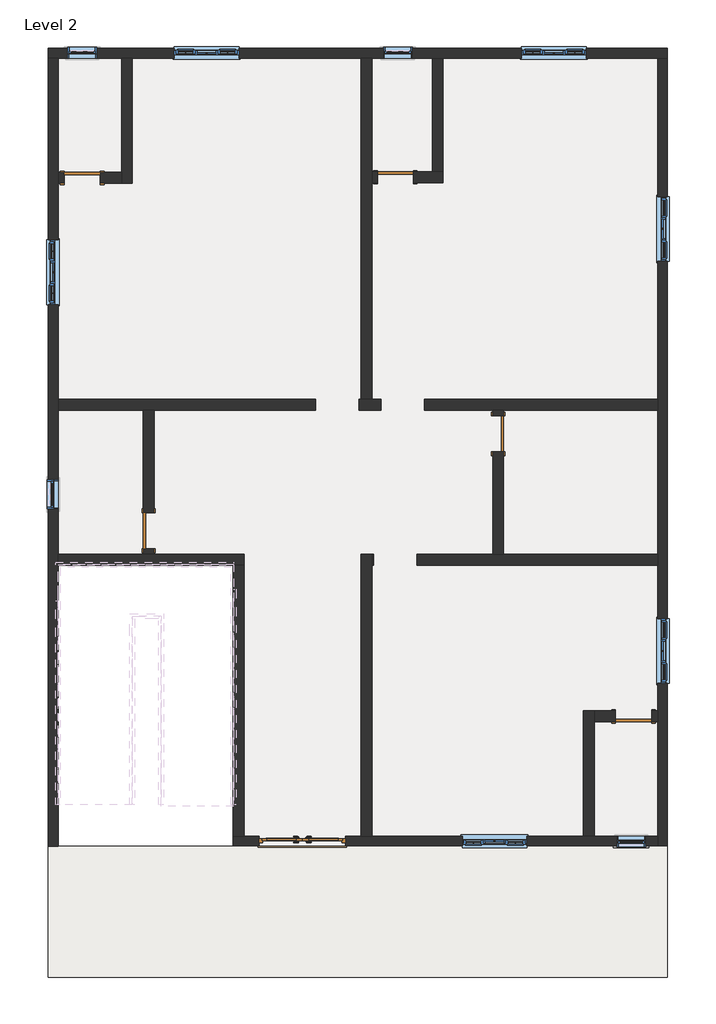
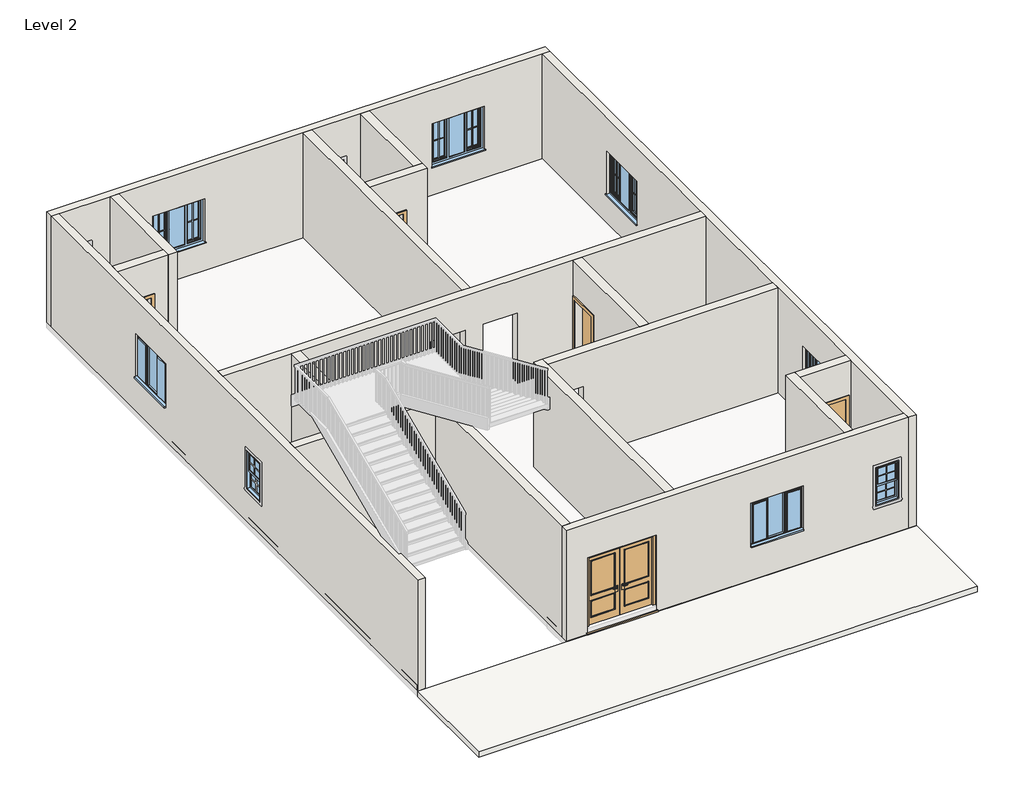
# One storey, part 1 of 4: 18 walls, 10 windows, 6 doors, 1 slab.
"""IFC4 building model written with IfcOpenShell, lengths in millimetres."""

from ifc_helpers import new_model, si_unit, frame, origin, place, context, project, spatial, polyline, outline, extrude, faceted_brep, transform, mapped, element, save
from components import doors_extdbl_2_1810x2110mm_9ab1935a, doors_extdbl_2_1810x2110mm_b7024f51, door_85036156, window_679d2811, windows_tpl_w_glazing_cross_bars_1360x1210mm_0306471f

model = new_model("IFC4")

# Units and contexts
model_context = context("Model", 3, world=origin())
ifc_project = project(units=[si_unit("LENGTHUNIT", "METRE", prefix="MILLI")], contexts=[model_context])

# Site, building, storey
site = spatial("IfcSite", under=ifc_project)
building = spatial("IfcBuilding", under=site)
storey = spatial("IfcBuildingStorey", under=building, Name="Level 2", Elevation=3048.0)

# Doors
placement = place(None, origin())
doors_extdbl_2_1810x2110mm_shape = doors_extdbl_2_1810x2110mm_9ab1935a(model_context)
doors_extdbl_2_1810x2110mm_2_shape = doors_extdbl_2_1810x2110mm_b7024f51(model_context)
element("IfcDoor", 1, ObjectType="Doors_ExtDbl_2 : 1810x2110mm", at=placement, inside=storey, context=model_context, shape_type="MappedRepresentation", body=[
    mapped(doors_extdbl_2_1810x2110mm_shape, transform((-2421.0852725, -7729.5064015, 3048.0), x_axis=(1.0, 0.0, 0.0), y_axis=(0.0, 1.0, 0.0), z_axis=(0.0, 0.0, 1.0))),
    mapped(doors_extdbl_2_1810x2110mm_2_shape, transform((-2421.0852725, -7729.5064015, 3048.0), x_axis=(1.0, 0.0, 0.0), y_axis=(0.0, 1.0, 0.0), z_axis=(0.0, 0.0, 1.0))),
])
door_shape = door_85036156(model_context)
element("IfcDoor", 2, ObjectType="Single-Flush : 30\" x 80\"", at=placement, inside=storey, context=model_context, shape_type="MappedRepresentation", body=[
    mapped(door_shape, transform((-7046.4415084, 6189.6935985, 3048.0), x_axis=(-1.0, 0.0, 0.0), y_axis=(0.0, -1.0, 0.0), z_axis=(0.0, 0.0, 1.0))),
])
element("IfcDoor", 3, ObjectType="Single-Flush : 30\" x 80\"", at=placement, inside=storey, context=model_context, shape_type="MappedRepresentation", body=[
    mapped(door_shape, transform((-467.8415084, 6203.2000968, 3048.0), x_axis=(-1.0, 0.0, 0.0), y_axis=(0.0, -1.0, 0.0), z_axis=(0.0, 0.0, 1.0))),
])
element("IfcDoor", 4, ObjectType="Single-Flush : 30\" x 80\"", at=placement, inside=storey, context=model_context, shape_type="MappedRepresentation", body=[
    mapped(door_shape, transform((-5649.4415084, -1217.2217109, 3048.0), x_axis=(0.0, -1.0, 0.0), y_axis=(1.0, 0.0, 0.0), z_axis=(0.0, 0.0, 1.0))),
])
element("IfcDoor", 5, ObjectType="Single-Flush : 30\" x 80\"", at=placement, inside=storey, context=model_context, shape_type="MappedRepresentation", body=[
    mapped(door_shape, transform((1691.1584916, 817.5935985, 3048.0), x_axis=(0.0, 1.0, 0.0), y_axis=(-1.0, 0.0, 0.0), z_axis=(0.0, 0.0, 1.0))),
])
element("IfcDoor", 6, ObjectType="Single-Flush : 30\" x 80\"", at=placement, inside=storey, context=model_context, shape_type="MappedRepresentation", body=[
    mapped(door_shape, transform((4535.9584916, -5113.3064015, 3048.0), x_axis=(1.0, 0.0, 0.0), y_axis=(0.0, 1.0, 0.0), z_axis=(0.0, 0.0, 1.0))),
])

# Slab
element("IfcSlab", 7, ObjectType="Generic - 12\"", at=placement, inside=storey, context=model_context, shape_type="SweptSolid", body=[
    extrude(outline(polyline([(5247.1584916, -7843.8064015), (5247.1584916, -10593.3139891), (-7757.6415084, -10593.3139891), (-7757.6415084, -7843.8064015), (5247.1584916, -7843.8064015)])), frame((0.0, 0.0, 2895.6), z_axis=(0.0, 0.0, 1.0), x_axis=(1.0, 0.0, 0.0)), (0.0, 0.0, 1.0), 152.4),
])

# Walls
element("IfcWall", 8, ObjectType="Generic - 4.5\"", at=placement, inside=storey, context=model_context, shape_type="Brep", body=[
    faceted_brep([(-1232.0415084, 1312.8935985, 5158.0), (-1232.0415084, 1312.8935985, 3048.0), (-770.4415084, 1312.8935985, 3048.0), (-770.4415084, 1312.8935985, 5158.0), (139.5584916, 1312.8935985, 5158.0), (139.5584916, 1312.8935985, 3048.0), (1576.8584916, 1312.8935985, 3048.0), (1805.4584916, 1312.8935985, 3048.0), (5043.9584916, 1312.8935985, 3048.0), (5043.9584916, 1312.8935985, 6096.0), (1805.4584916, 1312.8935985, 6096.0), (1576.8584916, 1312.8935985, 6096.0), (-5535.1415084, 1312.8935985, 6096.0), (-5763.7415084, 1312.8935985, 6096.0), (-7554.4415084, 1312.8935985, 6096.0), (-7554.4415084, 1312.8935985, 3048.0), (-5763.7415084, 1312.8935985, 3048.0), (-5535.1415084, 1312.8935985, 3048.0), (-2142.0415084, 1312.8935985, 3048.0), (-2142.0415084, 1312.8935985, 5158.0), (-770.4415084, 1541.4935985, 3048.0), (-963.1415084, 1541.4935985, 3048.0), (-1191.7415084, 1541.4935985, 3048.0), (-1232.0415084, 1541.4935985, 3048.0), (-1232.0415084, 1541.4935985, 5158.0), (-2142.0415084, 1541.4935985, 5158.0), (-2142.0415084, 1541.4935985, 3048.0), (-7554.4415084, 1541.4935985, 3048.0), (-7554.4415084, 1541.4935985, 6096.0), (-1191.7415084, 1541.4935985, 6096.0), (-963.1415084, 1541.4935985, 6096.0), (5043.9584916, 1541.4935985, 6096.0), (5043.9584916, 1541.4935985, 3048.0), (139.5584916, 1541.4935985, 3048.0), (139.5584916, 1541.4935985, 5158.0), (-770.4415084, 1541.4935985, 5158.0)], [[[0, 1, 2, 3, 4, 5, 6, 7, 8, 9, 10, 11, 12, 13, 14, 15, 16, 17, 18, 19]], [[20, 21, 22, 23, 24, 25, 26, 27, 28, 29, 30, 31, 32, 33, 34, 35]], [[33, 32, 8, 7, 6, 5]], [[2, 1, 23, 22, 21, 20]], [[18, 17, 16, 15, 27, 26]], [[14, 13, 12, 11, 10, 9, 31, 30, 29, 28]], [[9, 8, 32, 31]], [[15, 14, 28, 27]], [[5, 4, 34, 33]], [[3, 2, 20, 35]], [[4, 3, 35, 34]], [[26, 25, 19, 18]], [[24, 23, 1, 0]], [[25, 24, 0, 19]]]),
])
element("IfcWall", 9, ObjectType="Generic - 4.5\"", at=placement, inside=storey, context=model_context, shape_type="Brep", body=[
    faceted_brep([(-1191.7415084, 8704.2935985, 3048.0), (-1191.7415084, 1541.4935985, 3048.0), (-1191.7415084, 1541.4935985, 6096.0), (-1191.7415084, 8704.2935985, 6096.0), (-963.1415084, 8704.2935985, 3048.0), (-963.1415084, 8704.2935985, 6096.0), (-963.1415084, 6317.5000968, 6096.0), (-963.1415084, 6088.9000968, 6096.0), (-963.1415084, 1541.4935985, 6096.0), (-963.1415084, 1541.4935985, 3048.0), (-963.1415084, 6088.9000968, 3048.0), (-963.1415084, 6317.5000968, 3048.0)], [[[0, 1, 2, 3]], [[4, 5, 6, 7, 8, 9, 10, 11]], [[1, 0, 4, 11, 10, 9]], [[3, 2, 8, 7, 6, 5]], [[0, 3, 5, 4]], [[2, 1, 9, 8]]]),
])
element("IfcWall", 10, ObjectType="Generic - 4.5\"", at=placement, inside=storey, context=model_context, shape_type="Brep", body=[
    faceted_brep([(-6220.9415084, 8704.2935985, 3048.0), (-6220.9415084, 6303.9935985, 3048.0), (-6220.9415084, 6075.3935985, 3048.0), (-6220.9415084, 6075.3935985, 6096.0), (-6220.9415084, 6303.9935985, 6096.0), (-6220.9415084, 8704.2935985, 6096.0), (-5992.3415084, 8704.2935985, 3048.0), (-5992.3415084, 8704.2935985, 6096.0), (-5992.3415084, 6075.3935985, 6096.0), (-5992.3415084, 6075.3935985, 3048.0)], [[[0, 1, 2, 3, 4, 5]], [[6, 7, 8, 9]], [[2, 1, 0, 6, 9]], [[5, 4, 3, 8, 7]], [[0, 5, 7, 6]], [[3, 2, 9, 8]]]),
])
element("IfcWall", 11, ObjectType="Generic - 4.5\"", at=placement, inside=storey, context=model_context, shape_type="SweptSolid", body=[
    extrude(outline(polyline([(3048.0, -7554.4415084), (3048.0, -7427.4415084), (5080.0, -7427.4415084), (5080.0, -6665.4415084), (3048.0, -6665.4415084), (3048.0, -6220.9415084), (6096.0, -6220.9415084), (6096.0, -7554.4415084), (3048.0, -7554.4415084)])), frame((0.0, 6075.3935985, 0.0), z_axis=(0.0, 1.0, 0.0), x_axis=(0.0, 0.0, 1.0)), (0.0, 0.0, 1.0), 228.6),
])
element("IfcWall", 12, ObjectType="Generic - 4.5\"", at=placement, inside=storey, context=model_context, shape_type="Brep", body=[
    faceted_brep([(-963.1415084, 6088.9000968, 3048.0), (-848.8415084, 6088.9000968, 3048.0), (-848.8415084, 6088.9000968, 5080.0), (-86.8415084, 6088.9000968, 5080.0), (-86.8415084, 6088.9000968, 3048.0), (535.4584916, 6088.9000968, 3048.0), (535.4584916, 6088.9000968, 6096.0), (-963.1415084, 6088.9000968, 6096.0), (-848.8415084, 6317.5000968, 5080.0), (-848.8415084, 6317.5000968, 3048.0), (-963.1415084, 6317.5000968, 3048.0), (-963.1415084, 6317.5000968, 6096.0), (306.8584916, 6317.5000968, 6096.0), (535.4584916, 6317.5000968, 6096.0), (535.4584916, 6317.5000968, 3048.0), (306.8584916, 6317.5000968, 3048.0), (-86.8415084, 6317.5000968, 3048.0), (-86.8415084, 6317.5000968, 5080.0)], [[[0, 1, 2, 3, 4, 5, 6, 7]], [[8, 9, 10, 11, 12, 13, 14, 15, 16, 17]], [[10, 9, 1, 0]], [[16, 15, 14, 5, 4]], [[7, 6, 13, 12, 11]], [[0, 7, 11, 10]], [[6, 5, 14, 13]], [[2, 1, 9, 8]], [[3, 2, 8, 17]], [[4, 3, 17, 16]]]),
])
element("IfcWall", 13, ObjectType="Generic - 4.5\"", at=placement, inside=storey, context=model_context, shape_type="SweptSolid", body=[
    extrude(outline(polyline([(535.4584916, 8704.2935985), (535.4584916, 6317.5000968), (306.8584916, 6317.5000968), (306.8584916, 8704.2935985), (535.4584916, 8704.2935985)])), frame((0.0, 0.0, 3048.0), z_axis=(0.0, 0.0, 1.0), x_axis=(1.0, 0.0, 0.0)), (0.0, 0.0, 1.0), 3048.0),
])
element("IfcWall", 14, ObjectType="Generic - 4.5\"", at=placement, inside=storey, context=model_context, shape_type="SweptSolid", body=[
    extrude(outline(polyline([(-1598.2217109, 5080.0), (-1598.2217109, 3048.0), (-1712.5217109, 3048.0), (-1712.5217109, 6096.0), (1312.8935985, 6096.0), (1312.8935985, 3048.0), (-836.2217109, 3048.0), (-836.2217109, 5080.0), (-1598.2217109, 5080.0)])), frame((-5763.7415084, 0.0, 0.0), z_axis=(1.0, 0.0, 0.0), x_axis=(0.0, 1.0, 0.0)), (0.0, 0.0, 1.0), 228.6),
])
element("IfcWall", 15, ObjectType="Generic - 4.5\"", at=placement, inside=storey, context=model_context, shape_type="Brep", body=[
    faceted_brep([(-7554.4415084, -1941.1217109, 3048.0), (-3879.0290366, -1941.1217109, 3048.0), (-3650.4290366, -1941.1217109, 3048.0), (-3650.4290366, -1941.1217109, 6096.0), (-3879.0290366, -1941.1217109, 6096.0), (-7554.4415084, -1941.1217109, 6096.0), (-7554.4415084, -1712.5217109, 3048.0), (-7554.4415084, -1712.5217109, 6096.0), (-5763.7415084, -1712.5217109, 6096.0), (-5535.1415084, -1712.5217109, 6096.0), (-3650.4290366, -1712.5217109, 6096.0), (-3650.4290366, -1712.5217109, 3048.0), (-5535.1415084, -1712.5217109, 3048.0), (-5763.7415084, -1712.5217109, 3048.0)], [[[0, 1, 2, 3, 4, 5]], [[6, 7, 8, 9, 10, 11, 12, 13]], [[2, 1, 0, 6, 13, 12, 11]], [[5, 4, 3, 10, 9, 8, 7]], [[0, 5, 7, 6]], [[3, 2, 11, 10]]]),
])
element("IfcWall", 16, ObjectType="Generic - 4.5\"", at=placement, inside=storey, context=model_context, shape_type="SweptSolid", body=[
    extrude(outline(polyline([(-3879.0290366, -7627.9064015), (-3879.0290366, -1941.1217109), (-3650.4290366, -1941.1217109), (-3650.4290366, -7627.9064015), (-3879.0290366, -7627.9064015)])), frame((0.0, 0.0, 3048.0), z_axis=(0.0, 0.0, 1.0), x_axis=(1.0, 0.0, 0.0)), (0.0, 0.0, 1.0), 3048.0),
])
element("IfcWall", 17, ObjectType="Generic - 4.5\"", at=placement, inside=storey, context=model_context, shape_type="SweptSolid", body=[
    extrude(outline(polyline([(1312.8935985, 3048.0), (1198.5935985, 3048.0), (1198.5935985, 5080.0), (436.5935985, 5080.0), (436.5935985, 3048.0), (-1712.5217109, 3048.0), (-1712.5217109, 6096.0), (1312.8935985, 6096.0), (1312.8935985, 3048.0)])), frame((1576.8584916, 0.0, 0.0), z_axis=(1.0, 0.0, 0.0), x_axis=(0.0, 1.0, 0.0)), (0.0, 0.0, 1.0), 228.6),
])
element("IfcWall", 18, ObjectType="Generic - 4.5\"", at=placement, inside=storey, context=model_context, shape_type="Brep", body=[
    faceted_brep([(-963.1415084, -7627.9064015, 3048.0), (-963.1415084, -1941.1217109, 3048.0), (-963.1415084, -1712.5217109, 3048.0), (-963.1415084, -1712.5217109, 6096.0), (-963.1415084, -1941.1217109, 6096.0), (-963.1415084, -7627.9064015, 6096.0), (-1191.7415084, -7627.9064015, 3048.0), (-1191.7415084, -7627.9064015, 6096.0), (-1191.7415084, -1712.5217109, 6096.0), (-1191.7415084, -1712.5217109, 3048.0)], [[[0, 1, 2, 3, 4, 5]], [[6, 7, 8, 9]], [[2, 1, 0, 6, 9]], [[5, 4, 3, 8, 7]], [[0, 5, 7, 6]], [[3, 2, 9, 8]]]),
])
element("IfcWall", 19, ObjectType="Generic - 4.5\"", at=placement, inside=storey, context=model_context, shape_type="Brep", body=[
    faceted_brep([(-922.8415084, -1712.5217109, 5158.0), (-922.8415084, -1712.5217109, 3048.0), (-963.1415084, -1712.5217109, 3048.0), (-963.1415084, -1712.5217109, 6096.0), (1576.8584916, -1712.5217109, 6096.0), (1805.4584916, -1712.5217109, 6096.0), (5043.9584916, -1712.5217109, 6096.0), (5043.9584916, -1712.5217109, 3048.0), (1805.4584916, -1712.5217109, 3048.0), (1576.8584916, -1712.5217109, 3048.0), (-12.8415084, -1712.5217109, 3048.0), (-12.8415084, -1712.5217109, 5158.0), (-963.1415084, -1941.1217109, 3048.0), (-922.8415084, -1941.1217109, 3048.0), (-922.8415084, -1941.1217109, 5158.0), (-12.8415084, -1941.1217109, 5158.0), (-12.8415084, -1941.1217109, 3048.0), (5043.9584916, -1941.1217109, 3048.0), (5043.9584916, -1941.1217109, 6096.0), (-963.1415084, -1941.1217109, 6096.0)], [[[0, 1, 2, 3, 4, 5, 6, 7, 8, 9, 10, 11]], [[12, 13, 14, 15, 16, 17, 18, 19]], [[2, 1, 13, 12]], [[10, 9, 8, 7, 17, 16]], [[6, 5, 4, 3, 19, 18]], [[3, 2, 12, 19]], [[7, 6, 18, 17]], [[16, 15, 11, 10]], [[14, 13, 1, 0]], [[15, 14, 0, 11]]]),
])
element("IfcWall", 20, ObjectType="Generic - 4.5\"", at=placement, inside=storey, context=model_context, shape_type="Brep", body=[
    faceted_brep([(3710.4584916, -7627.9064015, 3048.0), (3710.4584916, -5227.6064015, 3048.0), (3710.4584916, -4999.0064015, 3048.0), (3710.4584916, -4999.0064015, 6096.0), (3710.4584916, -5227.6064015, 6096.0), (3710.4584916, -7627.9064015, 6096.0), (3481.8584916, -7627.9064015, 3048.0), (3481.8584916, -7627.9064015, 6096.0), (3481.8584916, -4999.0064015, 6096.0), (3481.8584916, -4999.0064015, 3048.0)], [[[0, 1, 2, 3, 4, 5]], [[6, 7, 8, 9]], [[2, 1, 0, 6, 9]], [[5, 4, 3, 8, 7]], [[0, 5, 7, 6]], [[3, 2, 9, 8]]]),
])
element("IfcWall", 21, ObjectType="Generic - 4.5\"", at=placement, inside=storey, context=model_context, shape_type="SweptSolid", body=[
    extrude(outline(polyline([(5080.0, 4916.9584916), (3048.0, 4916.9584916), (3048.0, 5043.9584916), (6096.0, 5043.9584916), (6096.0, 3710.4584916), (3048.0, 3710.4584916), (3048.0, 4154.9584916), (5080.0, 4154.9584916), (5080.0, 4916.9584916)])), frame((0.0, -5227.6064015, 0.0), z_axis=(0.0, 1.0, 0.0), x_axis=(0.0, 0.0, 1.0)), (0.0, 0.0, 1.0), 228.6),
])
element("IfcWall", 22, ObjectType="Generic - 9\"", at=placement, inside=storey, context=model_context, shape_type="Brep", body=[
    faceted_brep([(-7757.6415084, 8704.2935985, 3048.0), (-7554.4415084, 8704.2935985, 3048.0), (-6220.9415084, 8704.2935985, 3048.0), (-5992.3415084, 8704.2935985, 3048.0), (-1191.7415084, 8704.2935985, 3048.0), (-963.1415084, 8704.2935985, 3048.0), (306.8584916, 8704.2935985, 3048.0), (535.4584916, 8704.2935985, 3048.0), (5043.9584916, 8704.2935985, 3048.0), (5247.1584916, 8704.2935985, 3048.0), (5247.1584916, 8704.2935985, 6096.0), (5043.9584916, 8704.2935985, 6096.0), (535.4584916, 8704.2935985, 6096.0), (306.8584916, 8704.2935985, 6096.0), (-963.1415084, 8704.2935985, 6096.0), (-1191.7415084, 8704.2935985, 6096.0), (-5992.3415084, 8704.2935985, 6096.0), (-6220.9415084, 8704.2935985, 6096.0), (-7554.4415084, 8704.2935985, 6096.0), (-7757.6415084, 8704.2935985, 6096.0), (2179.5584916, 8704.2935985, 5172.4), (3539.5584916, 8704.2935985, 5172.4), (3539.5584916, 8704.2935985, 3962.4), (2179.5584916, 8704.2935985, 3962.4), (-5110.2415084, 8704.2935985, 5172.4), (-3750.2415084, 8704.2935985, 5172.4), (-3750.2415084, 8704.2935985, 3962.4), (-5110.2415084, 8704.2935985, 3962.4), (-7351.2415084, 8704.2935985, 5029.2), (-6741.6415084, 8704.2935985, 5029.2), (-6741.6415084, 8704.2935985, 3962.4), (-7351.2415084, 8704.2935985, 3962.4), (-721.8415084, 8704.2935985, 5029.2), (-112.2415084, 8704.2935985, 5029.2), (-112.2415084, 8704.2935985, 3962.4), (-721.8415084, 8704.2935985, 3962.4), (-7757.6415084, 8907.4935985, 3048.0), (-7757.6415084, 8907.4935985, 6096.0), (5247.1584916, 8907.4935985, 6096.0), (5247.1584916, 8907.4935985, 3048.0), (2179.5584916, 8907.4935985, 5172.4), (2179.5584916, 8907.4935985, 3962.4), (3539.5584916, 8907.4935985, 3962.4), (3539.5584916, 8907.4935985, 5172.4), (-5110.2415084, 8907.4935985, 5172.4), (-5110.2415084, 8907.4935985, 3962.4), (-3750.2415084, 8907.4935985, 3962.4), (-3750.2415084, 8907.4935985, 5172.4), (-7351.2415084, 8907.4935985, 5029.2), (-7351.2415084, 8907.4935985, 3962.4), (-6741.6415084, 8907.4935985, 3962.4), (-6741.6415084, 8907.4935985, 5029.2), (-721.8415084, 8907.4935985, 5029.2), (-721.8415084, 8907.4935985, 3962.4), (-112.2415084, 8907.4935985, 3962.4), (-112.2415084, 8907.4935985, 5029.2)], [[[0, 1, 2, 3, 4, 5, 6, 7, 8, 9, 10, 11, 12, 13, 14, 15, 16, 17, 18, 19], [20, 21, 22, 23], [24, 25, 26, 27], [28, 29, 30, 31], [32, 33, 34, 35]], [[36, 37, 38, 39], [40, 41, 42, 43], [44, 45, 46, 47], [48, 49, 50, 51], [52, 53, 54, 55]], [[9, 8, 7, 6, 5, 4, 3, 2, 1, 0, 36, 39]], [[19, 18, 17, 16, 15, 14, 13, 12, 11, 10, 38, 37]], [[10, 9, 39, 38]], [[41, 40, 20, 23]], [[42, 41, 23, 22]], [[43, 42, 22, 21]], [[40, 43, 21, 20]], [[45, 44, 24, 27]], [[46, 45, 27, 26]], [[47, 46, 26, 25]], [[44, 47, 25, 24]], [[49, 48, 28, 31]], [[50, 49, 31, 30]], [[51, 50, 30, 29]], [[48, 51, 29, 28]], [[53, 52, 32, 35]], [[54, 53, 35, 34]], [[55, 54, 34, 33]], [[52, 55, 33, 32]], [[0, 19, 37, 36]]]),
])
element("IfcWall", 23, ObjectType="Generic - 9\"", at=placement, inside=storey, context=model_context, shape_type="Brep", body=[
    faceted_brep([(5043.9584916, 8704.2935985, 3048.0), (5043.9584916, 1541.4935985, 3048.0), (5043.9584916, 1312.8935985, 3048.0), (5043.9584916, -1712.5217109, 3048.0), (5043.9584916, -1941.1217109, 3048.0), (5043.9584916, -4999.0064015, 3048.0), (5043.9584916, -5227.6064015, 3048.0), (5043.9584916, -7627.9064015, 3048.0), (5043.9584916, -7831.1064015, 3048.0), (5043.9584916, -7831.1064015, 6096.0), (5043.9584916, -7627.9064015, 6096.0), (5043.9584916, -5227.6064015, 6096.0), (5043.9584916, -4999.0064015, 6096.0), (5043.9584916, -1941.1217109, 6096.0), (5043.9584916, -1712.5217109, 6096.0), (5043.9584916, 1312.8935985, 6096.0), (5043.9584916, 1541.4935985, 6096.0), (5043.9584916, 8704.2935985, 6096.0), (5043.9584916, 5796.5435985, 5172.4), (5043.9584916, 4436.5435985, 5172.4), (5043.9584916, 4436.5435985, 3962.4), (5043.9584916, 5796.5435985, 3962.4), (5043.9584916, -3061.7064015, 5172.4), (5043.9584916, -4421.7064015, 5172.4), (5043.9584916, -4421.7064015, 3962.4), (5043.9584916, -3061.7064015, 3962.4), (5247.1584916, 8704.2935985, 3048.0), (5247.1584916, 8704.2935985, 6096.0), (5247.1584916, -7831.1064015, 6096.0), (5247.1584916, -7831.1064015, 3048.0), (5247.1584916, 5796.5435985, 5172.4), (5247.1584916, 5796.5435985, 3962.4), (5247.1584916, 4436.5435985, 3962.4), (5247.1584916, 4436.5435985, 5172.4), (5247.1584916, -3061.7064015, 5172.4), (5247.1584916, -3061.7064015, 3962.4), (5247.1584916, -4421.7064015, 3962.4), (5247.1584916, -4421.7064015, 5172.4)], [[[0, 1, 2, 3, 4, 5, 6, 7, 8, 9, 10, 11, 12, 13, 14, 15, 16, 17], [18, 19, 20, 21], [22, 23, 24, 25]], [[26, 27, 28, 29], [30, 31, 32, 33], [34, 35, 36, 37]], [[8, 7, 6, 5, 4, 3, 2, 1, 0, 26, 29]], [[17, 16, 15, 14, 13, 12, 11, 10, 9, 28, 27]], [[31, 30, 18, 21]], [[32, 31, 21, 20]], [[33, 32, 20, 19]], [[30, 33, 19, 18]], [[35, 34, 22, 25]], [[36, 35, 25, 24]], [[37, 36, 24, 23]], [[34, 37, 23, 22]], [[0, 17, 27, 26]], [[9, 8, 29, 28]]]),
])
element("IfcWall", 24, ObjectType="Generic - 9\"", at=placement, inside=storey, context=model_context, shape_type="Brep", body=[
    faceted_brep([(5043.9584916, -7627.9064015, 3048.0), (3710.4584916, -7627.9064015, 3048.0), (3481.8584916, -7627.9064015, 3048.0), (-963.1415084, -7627.9064015, 3048.0), (-1191.7415084, -7627.9064015, 3048.0), (-1516.0852725, -7627.9064015, 3048.0), (-1516.0852725, -7627.9064015, 5158.0), (-3326.0852725, -7627.9064015, 5158.0), (-3326.0852725, -7627.9064015, 3048.0), (-3650.4290366, -7627.9064015, 3048.0), (-3879.0290366, -7627.9064015, 3048.0), (-3879.0290366, -7627.9064015, 6096.0), (-3650.4290366, -7627.9064015, 6096.0), (-1191.7415084, -7627.9064015, 6096.0), (-963.1415084, -7627.9064015, 6096.0), (3481.8584916, -7627.9064015, 6096.0), (3710.4584916, -7627.9064015, 6096.0), (5043.9584916, -7627.9064015, 6096.0), (2294.9584916, -7627.9064015, 5172.4), (934.9584916, -7627.9064015, 5172.4), (934.9584916, -7627.9064015, 3962.4), (2294.9584916, -7627.9064015, 3962.4), (4789.9584916, -7627.9064015, 5029.2), (4180.3584916, -7627.9064015, 5029.2), (4180.3584916, -7627.9064015, 3962.4), (4789.9584916, -7627.9064015, 3962.4), (-1516.0852725, -7831.1064015, 5158.0), (-1516.0852725, -7831.1064015, 3048.0), (5043.9584916, -7831.1064015, 3048.0), (5043.9584916, -7831.1064015, 6096.0), (-3879.0290366, -7831.1064015, 6096.0), (-3879.0290366, -7831.1064015, 3048.0), (-3326.0852725, -7831.1064015, 3048.0), (-3326.0852725, -7831.1064015, 5158.0), (2294.9584916, -7831.1064015, 5172.4), (2294.9584916, -7831.1064015, 3962.4), (934.9584916, -7831.1064015, 3962.4), (934.9584916, -7831.1064015, 5172.4), (4789.9584916, -7831.1064015, 5029.2), (4789.9584916, -7831.1064015, 3962.4), (4180.3584916, -7831.1064015, 3962.4), (4180.3584916, -7831.1064015, 5029.2)], [[[0, 1, 2, 3, 4, 5, 6, 7, 8, 9, 10, 11, 12, 13, 14, 15, 16, 17], [18, 19, 20, 21], [22, 23, 24, 25]], [[26, 27, 28, 29, 30, 31, 32, 33], [34, 35, 36, 37], [38, 39, 40, 41]], [[32, 31, 10, 9, 8]], [[28, 27, 5, 4, 3, 2, 1, 0]], [[17, 16, 15, 14, 13, 12, 11, 30, 29]], [[11, 10, 31, 30]], [[35, 34, 18, 21]], [[36, 35, 21, 20]], [[37, 36, 20, 19]], [[34, 37, 19, 18]], [[39, 38, 22, 25]], [[40, 39, 25, 24]], [[41, 40, 24, 23]], [[38, 41, 23, 22]], [[8, 7, 33, 32]], [[6, 5, 27, 26]], [[7, 6, 26, 33]], [[0, 17, 29, 28]]]),
])
element("IfcWall", 25, ObjectType="Generic - 9\"", at=placement, inside=storey, context=model_context, shape_type="Brep", body=[
    faceted_brep([(-7757.6415084, 8704.2935985, 3048.0), (-7757.6415084, -7843.8064015, 3048.0), (-7757.6415084, -7843.8064015, 6096.0), (-7757.6415084, 8704.2935985, 6096.0), (-7757.6415084, 3528.4935985, 5172.4), (-7757.6415084, 3528.4935985, 3962.4), (-7757.6415084, 4888.4935985, 3962.4), (-7757.6415084, 4888.4935985, 5172.4), (-7757.6415084, -760.0217109, 5029.2), (-7757.6415084, -760.0217109, 3962.4), (-7757.6415084, -150.4217109, 3962.4), (-7757.6415084, -150.4217109, 5029.2), (-7554.4415084, 8704.2935985, 3048.0), (-7554.4415084, 8704.2935985, 6096.0), (-7554.4415084, 6303.9935985, 6096.0), (-7554.4415084, 6075.3935985, 6096.0), (-7554.4415084, 1541.4935985, 6096.0), (-7554.4415084, 1312.8935985, 6096.0), (-7554.4415084, -1712.5217109, 6096.0), (-7554.4415084, -1941.1217109, 6096.0), (-7554.4415084, -7843.8064015, 6096.0), (-7554.4415084, -7843.8064015, 3048.0), (-7554.4415084, -1941.1217109, 3048.0), (-7554.4415084, -1712.5217109, 3048.0), (-7554.4415084, 1312.8935985, 3048.0), (-7554.4415084, 1541.4935985, 3048.0), (-7554.4415084, 6075.3935985, 3048.0), (-7554.4415084, 6303.9935985, 3048.0), (-7554.4415084, 3528.4935985, 5172.4), (-7554.4415084, 4888.4935985, 5172.4), (-7554.4415084, 4888.4935985, 3962.4), (-7554.4415084, 3528.4935985, 3962.4), (-7554.4415084, -760.0217109, 5029.2), (-7554.4415084, -150.4217109, 5029.2), (-7554.4415084, -150.4217109, 3962.4), (-7554.4415084, -760.0217109, 3962.4)], [[[0, 1, 2, 3], [4, 5, 6, 7], [8, 9, 10, 11]], [[12, 13, 14, 15, 16, 17, 18, 19, 20, 21, 22, 23, 24, 25, 26, 27], [28, 29, 30, 31], [32, 33, 34, 35]], [[1, 0, 12, 27, 26, 25, 24, 23, 22, 21]], [[2, 1, 21, 20]], [[3, 2, 20, 19, 18, 17, 16, 15, 14, 13]], [[5, 4, 28, 31]], [[6, 5, 31, 30]], [[7, 6, 30, 29]], [[4, 7, 29, 28]], [[9, 8, 32, 35]], [[10, 9, 35, 34]], [[11, 10, 34, 33]], [[8, 11, 33, 32]], [[0, 3, 13, 12]]]),
])

# Windows
window_shape = window_679d2811(model_context)
element("IfcWindow", 26, ObjectType="Window-Double-Hung : 24\" x 42\"", at=placement, inside=storey, context=model_context, shape_type="MappedRepresentation", body=[
    mapped(window_shape, transform((-7656.0415084, -455.2217109, 3048.0), x_axis=(0.0, 1.0, 0.0), y_axis=(-1.0, 0.0, 0.0), z_axis=(0.0, 0.0, 1.0))),
])
element("IfcWindow", 27, ObjectType="Window-Double-Hung : 24\" x 42\"", at=placement, inside=storey, context=model_context, shape_type="MappedRepresentation", body=[
    mapped(window_shape, transform((-7046.4415084, 8805.8935985, 3048.0), x_axis=(1.0, 0.0, 0.0), y_axis=(0.0, 1.0, 0.0), z_axis=(0.0, 0.0, 1.0))),
])
element("IfcWindow", 28, ObjectType="Window-Double-Hung : 24\" x 42\"", at=placement, inside=storey, context=model_context, shape_type="MappedRepresentation", body=[
    mapped(window_shape, transform((-417.0415084, 8805.8935985, 3048.0), x_axis=(1.0, 0.0, 0.0), y_axis=(0.0, 1.0, 0.0), z_axis=(0.0, 0.0, 1.0))),
])
element("IfcWindow", 29, ObjectType="Window-Double-Hung : 24\" x 42\"", at=placement, inside=storey, context=model_context, shape_type="MappedRepresentation", body=[
    mapped(window_shape, transform((4485.1584916, -7729.5064015, 3048.0), x_axis=(-1.0, 0.0, 0.0), y_axis=(0.0, -1.0, 0.0), z_axis=(0.0, 0.0, 1.0))),
])
windows_tpl_w_glazing_cross_bars_1360x1210mm_shape = windows_tpl_w_glazing_cross_bars_1360x1210mm_0306471f(model_context)
element("IfcWindow", 30, ObjectType="Windows_Tpl_w-Glazing_Cross-Bars : 1360x1210mm", at=placement, inside=storey, context=model_context, shape_type="MappedRepresentation", body=[
    mapped(windows_tpl_w_glazing_cross_bars_1360x1210mm_shape, transform((5137.1019238, 4614.8769318, 3062.4), x_axis=(0.0, -1.0, 0.0), y_axis=(1.0, 0.0, 0.0), z_axis=(0.0, 0.0, 1.0))),
])
element("IfcWindow", 31, ObjectType="Windows_Tpl_w-Glazing_Cross-Bars : 1360x1210mm", at=placement, inside=storey, context=model_context, shape_type="MappedRepresentation", body=[
    mapped(windows_tpl_w_glazing_cross_bars_1360x1210mm_shape, transform((5137.1019238, -4243.3730682, 3062.4), x_axis=(0.0, -1.0, 0.0), y_axis=(1.0, 0.0, 0.0), z_axis=(0.0, 0.0, 1.0))),
])
element("IfcWindow", 32, ObjectType="Windows_Tpl_w-Glazing_Cross-Bars : 1360x1210mm", at=placement, inside=storey, context=model_context, shape_type="MappedRepresentation", body=[
    mapped(windows_tpl_w_glazing_cross_bars_1360x1210mm_shape, transform((1113.2918249, -7721.0498337, 3062.4), x_axis=(-1.0, 0.0, 0.0), y_axis=(0.0, -1.0, 0.0), z_axis=(0.0, 0.0, 1.0))),
])
element("IfcWindow", 33, ObjectType="Windows_Tpl_w-Glazing_Cross-Bars : 1360x1210mm", at=placement, inside=storey, context=model_context, shape_type="MappedRepresentation", body=[
    mapped(windows_tpl_w_glazing_cross_bars_1360x1210mm_shape, transform((3361.2251583, 8797.4370307, 3062.4), x_axis=(1.0, 0.0, 0.0), y_axis=(0.0, 1.0, 0.0), z_axis=(0.0, 0.0, 1.0))),
])
element("IfcWindow", 34, ObjectType="Windows_Tpl_w-Glazing_Cross-Bars : 1360x1210mm", at=placement, inside=storey, context=model_context, shape_type="MappedRepresentation", body=[
    mapped(windows_tpl_w_glazing_cross_bars_1360x1210mm_shape, transform((-3928.5748417, 8797.4370307, 3062.4), x_axis=(1.0, 0.0, 0.0), y_axis=(0.0, 1.0, 0.0), z_axis=(0.0, 0.0, 1.0))),
])
element("IfcWindow", 35, ObjectType="Windows_Tpl_w-Glazing_Cross-Bars : 1360x1210mm", at=placement, inside=storey, context=model_context, shape_type="MappedRepresentation", body=[
    mapped(windows_tpl_w_glazing_cross_bars_1360x1210mm_shape, transform((-7647.5849406, 4710.1602652, 3062.4), x_axis=(0.0, 1.0, 0.0), y_axis=(-1.0, 0.0, 0.0), z_axis=(0.0, 0.0, 1.0))),
])

save(model, "model.ifc")

# Revit data of these elements
# Type "Doors_ExtDbl_2 : 1810x2110mm"
#   Type Mark = "8"
#   Type Comments = "External Double"
#   Operation = "DoubleDoorSingleSwing"
#   Construction Type Id = "GSP4R"
#   Keynote = "L20"
#   Analytic Construction = "1/8 in Pilkington single glazing"
#   Wrap Layers (Int) from Ext = 0' - 6.98819"
#   Wrap Layers (Ext) from Ext = 0' - 4.03543"
#   Visual Light Transmittance = 0.9
#   Top of Lock Rail = 2' - 11.43307"
#   Thickness = 0' - 1.73228"
#   Stile Shutting = 0' - 4.92126"
#   Stile - Top Rail = 0' - 5.90551"
#   Stile - Lock Rail = 0' - 5.90551"
#   Stile - Hanging = 0' - 3.93701"
#   Stile - Bottom Rail = 0' - 11.81102"
#   Solar Heat Gain Coefficient = 0.78
#   Rough Width = 5' - 11.25984"
#   Rough Height = 6' - 11.07087"
#   O/A Frame Width = 0' - 2.51969"
#   Heat Transfer Coefficient (U) = 0.6496 BTU/(h·ft²·°F)
#   Handle Z Distance = 3' - 1.40157"
#   Glazing Thickness = 0' - 0.94488"
#   FrameWidth = 0' - 1.65354"
#   FrameOffset - External = 0' - 2.55906"
#   FrameDepth = 0' - 3.50394"
#   Door Panel Width = 2' - 9.54331"
#   Door Panel Thickness = 0' - 1.73228"
#   Door Panel Height = 6' - 6.74016"
#   Cill Thickness = 0' - 2.14567"
#   Cill Projection = 0' - 1.1811"
#   Handle X Distance = 0' - 2.95276"
#   Height = 6' - 11.07087"
#   Structural Tolerance = 0' - 0.25591"
#   Tolerance = 0' - 0.11811"
#   Undercut = 0' - 0.15748"
#   Width = 5' - 11.25984"
#   Cill Extension = 0' - 0.98425"
#   Cavity Closer Width = 0' - 1.9685"
#   Cavity Closer Offset from Ext = 0' - 4.03543"
#   Cavity Closer Depth = 0' - 3.34646"
#   Vis - Ironmongery = yes
#   Vis - Cavity Closers = yes
#   Define Thermal Properties by = 1
#   Function = 1
#   Material Glass = Door - Glazing
#   Handle Style = element 387460
#   Material Door = Door - Panel
#   Material Frame = Door - Frame/Mullion
#   Material Ironmongery = Door - Handle
#   Wall Closure = (empty or 0)
# Type "Single-Flush : 30\" x 80\""
#   Type Mark = "5"
#   Construction Type Id = "MDOOR"
#   Assembly Code = "C1020"
#   Analytic Construction = "Metal"
#   Thickness = 0' - 2"
#   Heat Transfer Coefficient (U) = 0.651978 BTU/(h·ft²·°F)
#   Height = 6' - 8"
#   Trim Projection Ext = 0' - 1"
#   Trim Projection Int = 0' - 1"
#   Trim Width = 0' - 3"
#   Width = 2' - 6"
#   Define Thermal Properties by = 1
#   Define Thermal Properties by = 1
#   Door Material = Door - Panel
#   Frame Material = Door - Frame
#   Visual Light Transmittance = 0
#   Solar Heat Gain Coefficient = 0
#   Function = (empty or 0)
#   Wall Closure = (empty or 0)
# Type "Generic - 12\""
#   Assembly Code = "B1010"
#   Function = 0
#   Layers, outside or top first: 0' - 6" no material (function 1)
# Type "Generic - 4.5\""
#   Assembly Code = "B2010"
#   Layers, outside or top first: 0' - 9" no material (function 1)
# Type "Generic - 9\""
#   Assembly Code = "B2010"
#   Layers, outside or top first: 0' - 8" no material (function 1)
# Type "Window-Double-Hung : 24\" x 42\""
#   Type Mark = "10"
#   Fire Rating = "0.5h"
#   Construction Type Id = "DG-DR"
#   Assembly Code = "B2020100"
#   Analytic Construction = "Double glazing - domestic"
#   Wall Thickness [instance default] = 0' - 6"
#   Window Inset [instance default] = 0' - 0"
#   Visual Light Transmittance = 0.81
#   Thermal Resistance (R) = 1.8146 (h·ft²·°F)/BTU
#   Solar Heat Gain Coefficient = 0.76
#   Muntin Width = 1' - 6"
#   Muntin Height = 1' - 5 1/8"
#   Interior Wall Closure [instance default] = 0' - 1 1/2"
#   Rough Width = 2' - 0 1/2"
#   Rough Height = 3' - 6 1/2"
#   Frame Extension [instance default] = 0' - 1 1/4"
#   Exterior Wall Closure [instance default] = 0' - 0 1/2"
#   Extension Jamb [instance default] = 0' - 1 1/2"
#   Heat Transfer Coefficient (U) = 0.5511 BTU/(h·ft²·°F)
#   Height = 3' - 6"
#   Width = 2' - 0"
#   Define Thermal Properties by = 1
#   Top Muntin Visibility = yes
#   Indicator Visibility [instance default] = yes
#   Extension Jamb Visibility [instance default] = yes
#   Interior Trim Visibility [instance default] = yes
#   Exterior Trim Visibility [instance default] = yes
#   Define Thermal Properties by = 1
#   Bottom Muntin Visibility = yes
#   Muntin Pattern = Muntin Pattern_2x2 : Muntin Pattern_2x2
#   Interior Trim Material = Wood - Stained
#   Interior Trim = Trim-Window-Interior-Flat : Picture Frame
#   Exterior Trim Material = Clad - White
#   Exterior Trim = Trim-Window-Exterior-Flat : with Sill
#   Glass Panel Material = Glass
#   Exterior Frame Material = Clad - White
#   Interior Frame Material = Wood - Stained
#   Wall Closure = (empty or 0)
# Type "Windows_Tpl_w-Glazing_Cross-Bars : 1360x1210mm"
#   Type Mark = "21"
#   Operation = "TriplePanelVertical"
#   Construction Type Id = "GSP4R"
#   Manufacturer = "Revit"
#   Keynote = "L10"
#   Analytic Construction = "1/8 in Pilkington single glazing"
#   Wrap Layers (Ext) from Ext = 0' - 4.03543"
#   Wrap Layers (Int) from Ext = 0' - 6.98819"
#   Window Board Projection = 0' - 0.98425"
#   Window Board Extension = 0' - 0.98425"
#   Visual Light Transmittance = 0.9
#   Solar Heat Gain Coefficient = 0.78
#   Rough Width = 4' - 5.54331"
#   Rough Height = 3' - 11.6378"
#   Height = 3' - 11.6378"
#   Width = 4' - 5.54331"
#   Heat Transfer Coefficient (U) = 0.6496 BTU/(h·ft²·°F)
#   Glazing Thickness = 0' - 0.94488"
#   Glazing Bar Thickness = 0' - 0.7874"
#   FrameOffset - External = 0' - 1.9685"
#   Frame Depth = 0' - 2.55906"
#   Default Head Height = 6' - 11.07087"
#   Cill Depth = 0' - 3.44488"
#   Cavity Closer Width = 0' - 1.9685"
#   Cavity Closer Offset from Ext = 0' - 4.03543"
#   Cavity Closer Depth = 0' - 3.34646"
#   Vis - Glazing Bars = yes
#   Vis - Cavity Closers = yes
#   Define Thermal Properties by = 1
#   Material Trim = Window Frame
#   Material Glazing Bars = Window Frame
#   Material Glass = Glass
#   Material Frame = Window Frame
#   Wall Closure = (empty or 0)
# Element 1 (IfcDoor, "Doors_ExtDbl_2 : 1810x2110mm")
#   Phase Created = New Construction
#   Materials on its faces: "Door - Panel", "Door - Handle", "Door - Frame/Mullion", "Door - Glazing"
# Elements 2, 3, 4, 5, 6 (IfcDoor, "Single-Flush : 30\" x 80\"")
#   Phase Created = New Construction
#   Materials on its faces: "Door - Frame", "Door - Panel"
# Element 7 (IfcSlab, "Generic - 12\"")
#   Height Offset From Level = 0' - 0"
#   Phase Created = New Construction
#   Materials on its faces: "Default Floor", "Concrete, Precast", "Default Mass Interior Wall"
# Elements 8, 9, 10, 11, 12, 13, 14, 17, 18, 19, 20, 21 (IfcWall, "Generic - 4.5\"")
#   Top Offset = 0' - 0"
#   Base Offset = 0' - 0"
#   wall height = 10' - 0"
#   Phase Created = New Construction
#   Base Constraint = Level 2
#   Top Constraint = Level 3
#   Materials on its faces: "Default Wall"
# Element 15 (IfcWall, "Generic - 4.5\"")
#   Top Offset = 0' - 0"
#   Base Offset = 0' - 0"
#   wall height = 10' - 0"
#   Phase Created = New Construction
#   Base Constraint = Level 2
#   Top Constraint = Level 3
#   Materials on its faces: "Default Wall", "Concrete, Precast"
# Element 16 (IfcWall, "Generic - 4.5\"")
#   Top Offset = 0' - 0"
#   Base Offset = 0' - 0"
#   wall height = 10' - 0"
#   Phase Created = New Construction
#   Base Constraint = Level 2
#   Top Constraint = Level 3
#   Materials on its faces: "Default Wall", "Bed-white fabric"
# Elements 22, 25 (IfcWall, "Generic - 9\"")
#   Top Offset = 0' - 0"
#   Base Offset = 0' - 0"
#   wall height = 10' - 0"
#   Phase Created = New Construction
#   Base Constraint = Level 2
#   Top Constraint = Level 3
#   Materials on its faces: "Default Wall", "Bed-white fabric"
# Element 23 (IfcWall, "Generic - 9\"")
#   Top Offset = 0' - 0"
#   Base Offset = 0' - 0"
#   wall height = 10' - 0"
#   Phase Created = New Construction
#   Base Constraint = Level 2
#   Top Constraint = Level 3
#   Materials on its faces: "Default Wall", "Bed-white fabric", "Bed-night tables"
# Element 24 (IfcWall, "Generic - 9\"")
#   Top Offset = 0' - 0"
#   Base Offset = 0' - 0"
#   wall height = 10' - 0"
#   Phase Created = New Construction
#   Base Constraint = Level 2
#   Top Constraint = Level 3
#   Materials on its faces: "Default Wall", "Bed-night tables", "Bed-white fabric"
# Element 26 (IfcWindow, "Window-Double-Hung : 24\" x 42\"")
#   Mark = "20"
#   Window Inset = 0' - 0"
#   Interior Wall Closure = 0' - 1 1/2"
#   Frame Extension = 0' - 1 1/4"
#   Exterior Wall Closure = 0' - 0 1/2"
#   Interior Trim Visibility = yes
#   Indicator Visibility = yes
#   Exterior Trim Visibility = yes
#   Phase Created = New Construction
#   Materials on its faces: "Wood - Stained", "Glass", "Clad - White"
# Element 27 (IfcWindow, "Window-Double-Hung : 24\" x 42\"")
#   Mark = "21"
#   Window Inset = 0' - 0"
#   Interior Wall Closure = 0' - 1 1/2"
#   Frame Extension = 0' - 1 1/4"
#   Exterior Wall Closure = 0' - 0 1/2"
#   Interior Trim Visibility = yes
#   Indicator Visibility = yes
#   Exterior Trim Visibility = yes
#   Phase Created = New Construction
#   Materials on its faces: "Wood - Stained", "Glass", "Clad - White"
# Element 28 (IfcWindow, "Window-Double-Hung : 24\" x 42\"")
#   Mark = "22"
#   Window Inset = 0' - 0"
#   Interior Wall Closure = 0' - 1 1/2"
#   Frame Extension = 0' - 1 1/4"
#   Exterior Wall Closure = 0' - 0 1/2"
#   Interior Trim Visibility = yes
#   Indicator Visibility = yes
#   Exterior Trim Visibility = yes
#   Phase Created = New Construction
#   Materials on its faces: "Wood - Stained", "Glass", "Clad - White"
# Element 29 (IfcWindow, "Window-Double-Hung : 24\" x 42\"")
#   Mark = "23"
#   Window Inset = 0' - 0"
#   Interior Wall Closure = 0' - 1 1/2"
#   Frame Extension = 0' - 1 1/4"
#   Exterior Wall Closure = 0' - 0 1/2"
#   Interior Trim Visibility = yes
#   Indicator Visibility = yes
#   Exterior Trim Visibility = yes
#   Phase Created = New Construction
#   Materials on its faces: "Wood - Stained", "Glass", "Clad - White"
# Element 30 (IfcWindow, "Windows_Tpl_w-Glazing_Cross-Bars : 1360x1210mm")
#   Mark = "14"
#   Phase Created = New Construction
#   Materials on its faces: "Window Frame", "Glass"
# Element 31 (IfcWindow, "Windows_Tpl_w-Glazing_Cross-Bars : 1360x1210mm")
#   Mark = "15"
#   Phase Created = New Construction
#   Materials on its faces: "Window Frame", "Glass"
# Element 32 (IfcWindow, "Windows_Tpl_w-Glazing_Cross-Bars : 1360x1210mm")
#   Mark = "16"
#   Phase Created = New Construction
#   Materials on its faces: "Window Frame", "Glass"
# Element 33 (IfcWindow, "Windows_Tpl_w-Glazing_Cross-Bars : 1360x1210mm")
#   Mark = "17"
#   Phase Created = New Construction
#   Materials on its faces: "Window Frame", "Glass"
# Element 34 (IfcWindow, "Windows_Tpl_w-Glazing_Cross-Bars : 1360x1210mm")
#   Mark = "18"
#   Phase Created = New Construction
#   Materials on its faces: "Window Frame", "Glass"
# Element 35 (IfcWindow, "Windows_Tpl_w-Glazing_Cross-Bars : 1360x1210mm")
#   Mark = "19"
#   Phase Created = New Construction
#   Materials on its faces: "Window Frame", "Glass"
# Materials
#   "Door - Glazing": colour RGB 0 0 255, transparency 0.75
#   "Door - Panel": class "Wood", colour RGB 210 159 95, transparency 0, Cost = 0
#   "Door - Frame/Mullion": class "Wood", colour RGB 212 179 113, transparency 0
#   "Door - Handle": colour RGB 247 247 247, transparency 0
#   "Door - Frame": colour RGB 118 70 51, transparency 0, Cost = 0
#   "Wood - Stained": class "Wood", colour RGB 224 178 126, transparency 0, Cost = 0
#   "Clad - White": class "Wood", colour RGB 242 242 238, transparency 0, Cost = 0
#   "Glass": class "Glass", colour RGB 0 128 192, transparency 0.75, Description = "Soda Lime Glass", Cost = 0
#   "Window Frame": colour RGB 249 249 249, transparency 0
#   "Default Floor": colour RGB 128 128 128, transparency 0, Cost = 0
#   "Concrete, Precast": class "Concrete", colour RGB 198 187 187, transparency 0, Description = "Precast concrete", Cost = 0
#   "Default Mass Interior Wall": class "Generic", colour RGB 195 229 126, transparency 0, Cost = 0
#   "Default Wall": colour RGB 128 128 128, transparency 0, Cost = 0
#   "Bed-white fabric": class "Paint", colour RGB 220 220 220, transparency 0
#   "Bed-night tables": class "Wood", colour RGB 38 33 19, transparency 0
